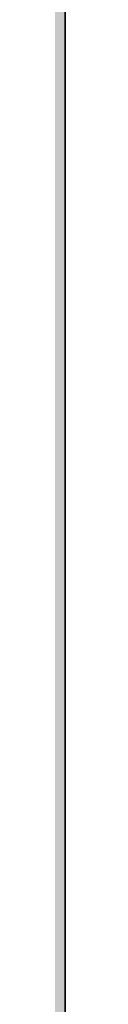
# Model space of a CAD drawing. Units: inches. Extents: x 2091 to 2899, y 967 to 2217.
# Tile 56 of 256: x 2212.14352 to 2212.1436, y 1099.95712 to 1099.99878. Entities that reach past the tile are written whole.
import ezdxf

# ---------------------------------------------------------------- set-up
doc = ezdxf.new("R2010")
doc.units = ezdxf.units.IN
doc.layers.add('A-WALL', color=7, linetype='Continuous', lineweight=35)
doc.layers.add('A-WALL-PATT', color=141, linetype='Continuous', lineweight=13, true_color=0xadddf7)

msp = doc.modelspace()

# ---------------------------------------------------------------- hatches: boundary and pattern name
at = {"layer": 'A-WALL-PATT'}
h = msp.add_hatch(color=256, dxfattribs=at)
h.dxf.hatch_style = 1
h.paths.add_polyline_path([(2212.143603, 1941.419059), (2387.643603, 1941.419059), (2387.643603, 1824.419059), (2392.143603, 1824.419059), (2392.143603, 1941.419059), (2609.643603, 1941.419059), (2609.643603, 1825.919059), (2614.143603, 1825.919059), (2614.143603, 1941.419059), (2794.143603, 1941.419059), (2794.143603, 1928.762166), (2803.143603, 1928.762166), (2803.143603, 2050.919059), (2203.143603, 2050.919059), (2203.143603, 1900.757859), (2212.143603, 1900.757859)])
h.paths.add_polyline_path([(2212.143603, 1945.919059), (2212.143603, 2041.919059), (2794.143603, 2041.919059), (2794.143603, 1945.919059), (2402.248245, 1945.919059), (2401.102434, 1945.775832), (2398.702434, 1945.775832)], flags=16)
h.paths.add_polyline_path([(2230.229861, 1948.062793), (2227.349861, 1949.502793), (2225.909861, 1951.902793), (2223.989861, 1952.862793), (2223.029861, 1955.262793), (2222.069861, 1959.582793), (2222.069861, 1963.422793), (2223.029861, 1965.662793), (2223.989861, 1965.342793), (2225.58591, 1963.860747), (2226.911533, 1964.957259), (2226.948861, 1965.938793), (2227.778319, 1966.952143), (2228.199916, 1968.878704), (2230.709861, 1964.862793), (2233.589861, 1966.302793), (2233.607309, 1966.331873), (2233.772659, 1964.938205), (2234.633802, 1963.676473), (2235.029861, 1963.902793), (2236.282035, 1965.572358), (2235.989861, 1962.942793), (2237.954512, 1957.540002), (2238.389861, 1957.902793), (2239.215861, 1960.305793), (2238.654565, 1966.38496), (2238.692792, 1966.438069), (2238.840578, 1967.499707), (2238.780291, 1967.687486), (2238.880538, 1967.786763), (2238.666861, 1966.251793), (2239.215861, 1960.305793), (2238.389861, 1957.902793), (2236.949861, 1956.702793), (2234.549861, 1949.982793)], flags=0)
h.paths.add_polyline_path([(2278.011974, 1948.062793), (2276.496427, 1947.873349), (2275.849833, 1947.688608), (2274.651974, 1947.102793)], flags=0)
h.paths.add_polyline_path([(2269.851974, 1955.742793), (2268.276176, 1956.629329), (2270.867302, 1956.348398), (2269.371974, 1958.142793), (2268.714964, 1959.192325), (2270.569833, 1958.728608), (2268.580725, 1961.906087), (2270.811974, 1960.891883), (2270.811974, 1963.422793), (2271.393315, 1964.779256), (2270.291762, 1966.156196), (2271.771974, 1965.662793), (2272.141387, 1966.524757), (2273.929833, 1965.928608), (2275.630385, 1968.054299), (2276.331938, 1966.72186), (2276.520431, 1966.952143), (2276.942029, 1968.878704), (2277.734293, 1967.611082), (2278.139888, 1969.46452), (2279.659124, 1967.033742), (2280.411974, 1966.782793), (2280.949302, 1967.588785), (2281.609833, 1967.368608), (2282.133266, 1968.153758), (2282.349235, 1966.333445), (2282.349849, 1966.332585), (2283.40755, 1968.09542), (2283.712631, 1965.52402), (2284.320221, 1964.633789), (2284.511809, 1964.889239), (2284.234974, 1965.704793), (2284.500472, 1967.318958), (2284.907944, 1965.41742), (2285.396313, 1966.068579), (2285.432833, 1966.290608), (2285.473338, 1966.171279), (2286.353919, 1967.345387), (2286.222007, 1966.158173), (2287.663492, 1968.080154), (2287.713974, 1968.442793), (2288.481599, 1969.016679), (2288.573993, 1968.728897), (2288.917461, 1969.06904), (2288.606833, 1966.837608), (2288.928726, 1963.35131), (2288.934974, 1963.356793), (2288.929731, 1963.340422), (2289.015281, 1962.413869), (2290.111223, 1963.875126), (2290.132833, 1963.942608), (2290.217672, 1964.017058), (2290.111223, 1963.875126), (2289.155833, 1960.891608), (2288.594036, 1959.257227), (2288.571974, 1959.102793), (2289.531974, 1960.542793), (2290.011974, 1962.462793), (2290.19184, 1962.642659), (2289.769833, 1959.688608), (2286.889833, 1957.288608), (2284.489833, 1950.568608), (2283.314658, 1950.046308), (2283.291974, 1949.982793), (2280.290059, 1948.648608), (2281.129833, 1948.648608), (2282.569833, 1948.168608), (2283.204726, 1948.062793), (2278.971974, 1948.062793), (2276.091974, 1949.502793), (2274.651974, 1951.902793), (2272.731974, 1952.862793)], flags=0)
h.paths.add_polyline_path([(2271.158868, 1958.021765), (2272.969833, 1955.848608), (2272.009833, 1960.168608), (2272.009833, 1964.008608), (2272.624426, 1965.442658), (2274.328023, 1963.860747), (2275.653646, 1964.957259), (2275.637743, 1964.53909), (2277.412231, 1966.006888), (2277.032974, 1965.156793), (2276.829924, 1964.975597), (2276.766012, 1963.295014), (2277.449635, 1962.66022), (2279.451974, 1964.862793), (2282.331974, 1966.302793), (2283.529833, 1966.888608), (2283.294512, 1966.770948), (2283.912993, 1963.8847), (2284.899249, 1964.448275), (2284.731974, 1962.942793), (2286.696625, 1957.540002), (2287.131974, 1957.902793), (2287.541913, 1959.095388), (2287.779395, 1958.442311), (2285.682738, 1956.695097), (2285.876503, 1959.795336), (2284.731974, 1962.942793), (2284.899249, 1964.448275), (2283.912993, 1963.8847), (2284.223833, 1962.434116), (2283.424365, 1963.605484), (2281.609833, 1962.568608), (2281.129833, 1960.168608), (2282.089833, 1956.328608), (2283.049833, 1952.968608), (2282.569833, 1950.568608), (2280.169833, 1948.648608), (2279.883316, 1948.791867), (2278.971974, 1948.062793), (2278.971974, 1949.022793), (2278.672313, 1949.397368), (2277.289833, 1950.088608), (2275.849833, 1952.488608), (2273.929833, 1953.448608), (2272.489833, 1954.888608), (2271.921647, 1954.888608), (2271.771974, 1955.262793)], flags=0)
h.paths.add_polyline_path([(2311.994146, 1955.742793), (2312.062717, 1955.674221), (2312.0551, 1955.7085)], flags=0)
h.paths.add_polyline_path([(2331.956146, 1963.951793), (2333.396146, 1965.391793), (2331.077146, 1963.356793), (2330.998603, 1963.111517)], flags=0)
h.paths.add_polyline_path([(2310.554146, 1954.302793), (2307.039807, 1956.279943), (2310.762903, 1955.876284), (2312.474146, 1953.822793), (2313.434146, 1951.422793), (2315.354146, 1950.462793), (2316.794146, 1948.062793), (2317.466146, 1947.726793), (2319.368691, 1947.964611), (2317.754146, 1949.982793), (2317.569531, 1950.610485), (2316.794146, 1951.902793), (2314.874146, 1952.862793), (2313.914146, 1955.262793), (2311.514146, 1958.142793), (2309.375489, 1961.559168), (2311.514146, 1960.337078), (2311.514146, 1961.982793), (2310.604672, 1963.119635), (2311.726605, 1962.47853), (2312.418332, 1964.09256), (2312.255964, 1964.29552), (2313.194146, 1963.982793), (2313.914146, 1965.662793), (2314.646778, 1965.418582), (2315.354146, 1966.302793), (2316.794146, 1967.742793), (2316.157435, 1966.946904), (2317.034111, 1965.28186), (2317.222604, 1965.512143), (2317.777048, 1968.045771), (2318.474111, 1966.72186), (2318.662604, 1966.952143), (2319.084201, 1968.878704), (2321.207049, 1965.482147), (2322.161419, 1966.913702), (2322.554146, 1966.782793), (2322.785988, 1967.130555), (2322.881646, 1966.324293), (2323.312041, 1965.72174), (2323.651289, 1965.891364), (2324.3965, 1967.133382), (2324.656945, 1964.938205), (2324.971986, 1964.476611), (2325.38728, 1967.001499), (2325.940813, 1964.418348), (2327.228929, 1966.135836), (2327.16632, 1965.572358), (2328.059139, 1966.762783), (2328.224576, 1966.247486), (2329.667971, 1967.67691), (2329.664576, 1967.687486), (2329.764823, 1967.786763), (2329.551146, 1966.251793), (2330.100146, 1960.305793), (2329.332814, 1958.07347), (2329.313065, 1957.935225), (2329.634146, 1958.202793), (2330.234146, 1959.102793), (2330.714146, 1961.022793), (2331.034146, 1961.342793), (2330.714146, 1959.102793), (2329.634146, 1958.202793), (2329.274146, 1957.662793), (2327.712112, 1956.361098), (2325.434146, 1949.982793), (2324.333769, 1949.493736), (2323.994146, 1948.542793), (2319.674146, 1946.622793), (2316.794146, 1948.062793), (2315.354146, 1950.462793), (2313.434146, 1951.422793)], flags=0)
h.paths.add_polyline_path([(2321.335684, 1947.952023), (2321.114146, 1948.062793), (2321.114146, 1949.022793), (2319.194146, 1951.422793), (2316.794146, 1959.582793), (2316.663237, 1959.582793), (2315.354146, 1958.142793), (2314.394146, 1958.142793), (2313.148303, 1958.709085), (2312.954146, 1959.582793), (2312.954146, 1960.891883), (2315.834146, 1959.582793), (2316.663237, 1959.582793), (2317.314709, 1960.299412), (2315.030195, 1962.420747), (2316.355818, 1963.517259), (2316.372337, 1963.951615), (2316.470195, 1963.860747), (2317.795818, 1964.957259), (2317.755219, 1963.889687), (2319.175146, 1965.156793), (2319.498407, 1965.881372), (2321.114146, 1965.342793), (2323.235885, 1962.372358), (2325.686349, 1963.772623), (2325.542789, 1962.480576), (2325.198783, 1963.494014), (2324.47851, 1963.082429), (2324.926005, 1960.994116), (2324.078087, 1962.236473), (2322.414791, 1961.286018), (2322.074146, 1959.582793), (2323.034146, 1955.742793), (2323.994146, 1952.382793), (2323.514146, 1949.982793), (2322.142717, 1948.88565), (2322.074146, 1948.542793)], flags=0)
h.paths.add_polyline_path([(2320.207479, 1963.337459), (2320.154146, 1963.422793), (2320.394146, 1963.542793)], flags=0)
h.paths.add_polyline_path([(2353.850527, 1965.8105), (2354.030527, 1965.7505), (2354.330527, 1966.4505), (2354.330527, 1966.9305)], flags=0)
h.paths.add_polyline_path([(2359.020582, 1969.026412), (2359.098382, 1968.901932), (2359.233527, 1969.5195), (2359.233527, 1969.9995)], flags=0)
h.paths.add_polyline_path([(2358.256694, 1966.681672), (2357.983601, 1966.348035), (2358.211267, 1966.146175), (2358.410492, 1966.389568)], flags=0)
h.paths.add_polyline_path([(2357.768473, 1966.058778), (2357.7322, 1965.104967), (2357.751047, 1965.120556), (2357.769527, 1965.6065), (2357.769527, 1966.057843)], flags=0)
h.paths.add_polyline_path([(2359.111527, 1965.3045), (2359.111527, 1964.8245), (2359.844527, 1966.4675), (2359.844527, 1966.9475)], flags=0)
h.paths.add_polyline_path([(2360.223684, 1966.621449), (2360.698527, 1969.3625), (2360.698527, 1969.8425), (2360.210527, 1967.0255), (2360.210527, 1966.6425)], flags=0)
h.paths.add_polyline_path([(2363.450527, 1967.8905), (2363.450527, 1968.3705), (2362.490527, 1966.9305), (2362.656045, 1966.698776)], flags=0)
h.paths.add_polyline_path([(2364.475523, 1966.078826), (2365.850527, 1968.3705), (2365.850527, 1968.8505), (2364.427975, 1966.479581)], flags=0)
h.paths.add_polyline_path([(2366.313527, 1965.8525), (2366.366709, 1965.695829), (2366.802527, 1968.3455), (2366.802527, 1968.8255)], flags=0)
h.paths.add_polyline_path([(2367.16531, 1965.803544), (2367.290527, 1966.9305), (2367.290527, 1967.4105), (2367.102701, 1965.720066)], flags=0)
h.paths.add_polyline_path([(2370.036527, 1959.9735), (2371.013527, 1963.0245), (2371.013527, 1963.5045), (2370.036527, 1960.4535)], flags=0)
h.paths.add_polyline_path([(2371.610527, 1960.2105), (2372.570527, 1961.6505), (2372.570527, 1962.1305), (2371.802527, 1960.9785)], flags=0)
h.paths.add_polyline_path([(2350.873666, 1956.005086), (2351.930527, 1955.8905), (2354.490527, 1953.3305), (2353.850527, 1954.9305), (2351.450527, 1957.8105), (2347.935527, 1963.4255), (2347.935527, 1963.9055), (2351.450527, 1958.2905), (2353.705073, 1955.585046), (2352.890527, 1959.2505), (2352.890527, 1959.7305), (2352.890527, 1961.924786), (2356.730527, 1959.7305), (2358.454471, 1961.626838), (2354.810527, 1965.0105), (2355.030855, 1965.28591), (2358.691091, 1961.88712), (2361.530527, 1965.0105), (2364.376495, 1966.433484), (2364.524394, 1965.186911), (2365.454468, 1963.824181), (2365.881073, 1964.067955), (2365.370527, 1966.4505), (2365.370527, 1966.9305), (2366.810527, 1960.2105), (2366.810527, 1959.7305), (2366.388709, 1952.981409), (2367.770527, 1956.8505), (2368.641225, 1957.576082), (2366.810527, 1962.6105), (2366.810527, 1963.0905), (2368.775179, 1957.68771), (2369.210527, 1958.0505), (2370.001592, 1960.351867), (2369.475232, 1966.052668), (2369.513458, 1966.105777), (2369.514173, 1966.110912), (2369.475232, 1966.532668), (2369.513458, 1966.585777), (2369.614635, 1967.312591), (2369.182527, 1968.6585), (2369.182527, 1969.1385), (2369.600957, 1967.835194), (2369.701204, 1967.934471), (2369.717947, 1968.054743), (2370.145176, 1968.374145), (2369.778707, 1968.011224), (2369.701204, 1967.454471), (2370.468161, 1968.214004), (2369.674936, 1967.265771), (2369.514173, 1966.110912), (2370.036527, 1960.4535), (2370.036527, 1959.9735), (2369.441756, 1958.243191), (2370.650527, 1959.2505), (2371.045821, 1962.017559), (2371.130527, 1962.1305), (2370.650527, 1958.7705), (2367.770527, 1956.3705), (2365.370527, 1949.6505), (2362.079099, 1948.187643), (2363.450527, 1947.7305), (2361.050527, 1947.7305), (2360.090527, 1947.7305), (2357.103861, 1947.357167), (2360.090527, 1948.2105), (2358.170527, 1949.1705), (2356.730527, 1951.5705), (2354.810527, 1952.5305), (2351.930527, 1955.4105)], flags=0)
h.paths.add_polyline_path([(2361.050527, 1948.6905), (2359.130527, 1951.0905), (2356.730527, 1959.2505), (2355.770527, 1959.2505), (2352.890527, 1960.559591), (2352.890527, 1961.444786), (2355.890527, 1959.7305), (2356.730527, 1959.7305), (2356.837194, 1959.367834), (2361.530527, 1964.5305), (2363.248422, 1965.389448), (2364.92531, 1963.041805), (2362.490527, 1961.6505), (2362.063861, 1959.517167), (2362.970527, 1955.8905), (2363.930527, 1952.5305), (2363.930527, 1952.0505), (2363.450527, 1949.6505), (2361.050527, 1947.7305)], flags=0)
h.paths.add_polyline_path([(2359.130527, 1951.5705), (2359.290527, 1951.3705), (2361.050527, 1954.4505), (2361.050527, 1954.9305)], flags=0)
h.paths.add_polyline_path([(2357.219527, 1966.5455), (2356.792527, 1968.8145), (2356.792527, 1969.2945), (2357.219527, 1967.0255)], flags=0)
h.paths.add_polyline_path([(2361.050527, 1954.4505), (2361.530527, 1958.7705), (2361.530527, 1959.2505), (2361.050527, 1954.9305)], flags=0)
h.paths.add_polyline_path([(2402.548287, 1948.486076), (2402.302434, 1948.415832), (2402.590434, 1948.415832)], flags=0)
h.paths.add_polyline_path([(2394.142434, 1956.095832), (2395.685052, 1954.553214), (2396.720495, 1953.970679), (2396.062434, 1955.615832), (2395.241381, 1956.601096), (2395.878904, 1956.441715), (2395.102434, 1959.935832), (2395.102434, 1963.775832), (2396.062434, 1966.015832), (2397.022434, 1965.695832), (2398.618483, 1964.213787), (2399.944106, 1965.310299), (2399.981434, 1966.291832), (2400.810891, 1967.305183), (2401.232489, 1969.231744), (2403.537949, 1965.543008), (2403.941984, 1967.389316), (2404.702434, 1967.135832), (2405.460328, 1966.07478), (2406.622434, 1966.655832), (2406.639882, 1966.684913), (2406.805232, 1965.291245), (2406.925694, 1965.114746), (2407.342434, 1964.975832), (2407.874326, 1965.77367), (2408.1691, 1964.398055), (2409.314608, 1965.925398), (2409.217458, 1965.051054), (2409.445232, 1963.131245), (2410.306374, 1961.869513), (2410.702434, 1962.095832), (2411.442269, 1963.082279), (2411.165434, 1963.897832), (2411.616426, 1966.639757), (2411.725365, 1966.791109), (2411.873151, 1967.852747), (2411.812864, 1968.040526), (2411.913111, 1968.139803), (2411.699434, 1966.604832), (2412.248434, 1960.658832), (2413.225434, 1963.709832), (2414.3779, 1964.72116), (2414.513151, 1965.692747), (2414.452864, 1965.880526), (2414.553111, 1965.979803), (2414.3779, 1964.72116), (2414.519817, 1964.845697), (2414.365365, 1964.631109), (2414.339434, 1964.444832), (2414.888434, 1958.498832), (2414.062434, 1956.095832), (2412.622434, 1954.895832), (2410.17137, 1948.032854), (2410.016719, 1948.084404), (2405.902434, 1946.255832), (2405.902434, 1947.215832), (2405.204252, 1948.08856), (2404.222434, 1948.415832), (2403.262434, 1948.415832), (2400.382434, 1949.855832), (2399.662434, 1951.055832), (2397.982434, 1952.735832), (2397.022434, 1953.215832), (2395.685052, 1954.553214), (2392.656776, 1956.256908)], flags=0)
h.paths.add_polyline_path([(2409.08565, 1964.407441), (2409.130363, 1964.275715), (2409.262434, 1964.495832)], flags=0)
h.paths.add_polyline_path([(2397.742434, 1961.615832), (2398.702434, 1963.855832), (2399.662434, 1963.535832), (2401.426563, 1965.740994), (2401.791415, 1966.5588), (2402.071434, 1965.070832), (2402.835507, 1964.393367), (2403.262398, 1964.9149), (2403.338119, 1964.771086), (2402.615516, 1963.976223), (2402.498612, 1960.902238), (2403.542997, 1959.932452), (2404.413203, 1960.889679), (2404.702434, 1962.335832), (2407.916347, 1964.172354), (2409.520211, 1961.926944), (2410.987085, 1957.893042), (2411.422434, 1958.255832), (2412.047964, 1960.075625), (2412.410341, 1959.079088), (2411.675621, 1958.466821), (2411.662434, 1958.255832), (2411.62607, 1958.425529), (2409.982434, 1957.055832), (2407.582434, 1950.335832), (2403.262434, 1948.415832), (2403.262434, 1949.375832), (2401.342434, 1951.775832), (2399.416508, 1958.323981), (2397.742434, 1959.084923), (2397.742434, 1959.970118), (2397.102434, 1960.335832), (2397.742434, 1960.044923)], flags=0)
h.paths.add_polyline_path([(2405.902434, 1952.975832), (2405.950434, 1953.407832), (2406.016719, 1953.175832)], flags=0)
h.paths.add_polyline_path([(2449.817778, 1967.114014), (2449.752323, 1967.135832), (2449.793703, 1967.077901)], flags=0)
h.paths.add_polyline_path([(2451.697696, 1966.61812), (2451.740895, 1966.690118), (2451.692051, 1966.665696)], flags=0)
h.paths.add_polyline_path([(2454.343628, 1965.737572), (2455.752323, 1967.615832), (2455.992323, 1968.095832), (2454.364497, 1965.925398)], flags=0)
h.paths.add_polyline_path([(2457.547323, 1968.863832), (2457.787323, 1969.343832), (2457.054323, 1968.795832), (2457.007622, 1968.460345)], flags=0)
h.paths.add_polyline_path([(2456.921784, 1967.856662), (2456.802238, 1968.229016), (2456.723, 1967.659803)], flags=0)
h.paths.add_polyline_path([(2457.302323, 1967.376832), (2457.542323, 1967.856832), (2456.810323, 1966.839832), (2456.740516, 1966.700218), (2456.749021, 1966.608105)], flags=0)
h.paths.add_polyline_path([(2458.275323, 1963.709832), (2458.155343, 1963.335153), (2460.354323, 1965.264832), (2460.594323, 1965.744832)], flags=0)
h.paths.add_polyline_path([(2458.392323, 1962.815832), (2458.364088, 1962.618185), (2459.592323, 1964.255832), (2459.832323, 1964.735832)], flags=0)
h.paths.add_polyline_path([(2459.352323, 1962.815832), (2459.272323, 1962.495832), (2460.072323, 1963.295832), (2460.312323, 1963.775832)], flags=0)
h.paths.add_polyline_path([(2458.680323, 1960.607832), (2458.632323, 1960.415832), (2459.592323, 1961.855832), (2459.832323, 1962.335832)], flags=0)
h.paths.add_polyline_path([(2437.83817, 1956.24265), (2439.192323, 1956.095832), (2441.352323, 1953.935832), (2440.872323, 1955.135832), (2438.472323, 1958.015832), (2438.071563, 1958.656023), (2438.712323, 1958.495832), (2440.639596, 1956.183105), (2439.912323, 1959.455832), (2439.912323, 1963.295832), (2441.352323, 1966.655832), (2441.592323, 1967.135832), (2441.112323, 1966.015832), (2442.072323, 1965.695832), (2443.988993, 1968.09167), (2444.241323, 1966.750832), (2444.916801, 1966.15192), (2445.676574, 1967.080136), (2446.255323, 1969.724832), (2446.495323, 1970.204832), (2446.282379, 1969.231744), (2447.362672, 1967.503275), (2447.720323, 1969.567832), (2447.960323, 1970.047832), (2447.48548, 1967.306781), (2448.792323, 1965.215832), (2448.472323, 1964.863832), (2448.552323, 1964.735832), (2451.452051, 1966.185696), (2451.615122, 1964.811245), (2452.307917, 1963.796172), (2453.234505, 1964.325651), (2454.072323, 1960.415832), (2453.628687, 1953.317651), (2454.792323, 1956.575832), (2455.032323, 1957.055832), (2455.718835, 1957.627926), (2453.832323, 1962.815832), (2453.940966, 1963.793615), (2453.335323, 1965.577832), (2453.824323, 1968.550832), (2454.064323, 1969.030832), (2453.575323, 1966.057832), (2454.040333, 1964.687919), (2453.832323, 1962.815832), (2455.718835, 1957.627926), (2456.367207, 1958.168235), (2457.058323, 1960.178832), (2457.298323, 1960.658832), (2456.472323, 1958.255832), (2457.717729, 1959.29367), (2457.672323, 1958.975832), (2454.889951, 1956.657188), (2453.614142, 1953.084923), (2453.592323, 1952.735832), (2453.352323, 1952.255832), (2453.359596, 1952.372196), (2452.632323, 1950.335832), (2452.392323, 1949.855832), (2449.203752, 1948.43869), (2450.712323, 1947.935832), (2448.072323, 1947.935832), (2447.112323, 1947.935832), (2444.552323, 1947.615832), (2447.199596, 1948.372196), (2445.192323, 1949.375832), (2443.752323, 1951.775832), (2441.832323, 1952.735832), (2438.952323, 1955.615832)], flags=0)
h.paths.add_polyline_path([(2443.992323, 1959.935832), (2444.040323, 1959.772632), (2444.121554, 1959.861986)], flags=0)
h.paths.add_polyline_path([(2442.912323, 1959.935832), (2443.032323, 1959.935832), (2442.445657, 1960.202499)], flags=0)
h.paths.add_polyline_path([(2444.982943, 1965.019677), (2445.279323, 1965.264832), (2445.519323, 1965.744832), (2444.993996, 1965.310299)], flags=0)
h.paths.add_polyline_path([(2446.133323, 1965.029832), (2446.330366, 1965.471499), (2444.970323, 1964.257832), (2444.730323, 1963.777832)], flags=0)
h.paths.add_polyline_path([(2442.792323, 1959.455832), (2443.752323, 1959.455832), (2446.152323, 1951.295832), (2446.412323, 1951.750832), (2446.392323, 1951.775832), (2448.080599, 1954.730315), (2448.552323, 1958.975832), (2441.832323, 1965.215832), (2442.154946, 1965.619111), (2448.792323, 1959.455832), (2448.312323, 1955.135832), (2448.072323, 1954.655832), (2446.412323, 1951.750832), (2448.312323, 1949.375832), (2448.312323, 1948.415832), (2450.540895, 1950.19869), (2450.952323, 1952.255832), (2449.992323, 1955.615832), (2449.032323, 1959.455832), (2449.512323, 1961.855832), (2449.752323, 1962.335832), (2449.674904, 1961.948736), (2452.994505, 1963.845651), (2453.064414, 1963.519409), (2452.884611, 1963.782854), (2449.674904, 1961.948736), (2449.272323, 1959.935832), (2450.232323, 1956.095832), (2451.192323, 1952.735832), (2450.712323, 1950.335832), (2450.472323, 1949.855832), (2448.072323, 1947.935832), (2448.072323, 1948.535832), (2445.432323, 1949.855832), (2443.992323, 1952.255832), (2442.072323, 1953.215832), (2441.112323, 1955.615832), (2440.152323, 1959.935832), (2440.152323, 1960.655832)], flags=0)
h.paths.add_polyline_path([(2456.692323, 1966.985832), (2457.608323, 1968.080832), (2457.848323, 1968.560832), (2456.932323, 1967.465832)], flags=0)
h.paths.add_polyline_path([(2489.89657, 1966.580241), (2489.942948, 1966.189347), (2490.747488, 1967.530248), (2491.319122, 1968.951161)], flags=0)
h.paths.add_polyline_path([(2473.562471, 1956.407131), (2477.139981, 1956.019257), (2476.955333, 1956.240834), (2475.108049, 1957.280108), (2476.347488, 1956.970248), (2475.186901, 1958.824216), (2476.919122, 1958.391161), (2475.411642, 1960.799269), (2477.787488, 1959.719339), (2477.787488, 1962.250248), (2477.637399, 1962.43786), (2477.82255, 1962.332059), (2478.359122, 1963.58406), (2478.359122, 1963.671161), (2477.324348, 1964.964628), (2478.714826, 1964.501135), (2479.319122, 1965.911161), (2480.279122, 1965.591161), (2481.783965, 1967.472214), (2482.116488, 1965.705248), (2482.880562, 1965.027782), (2483.209305, 1965.429408), (2483.220169, 1965.71509), (2483.07594, 1965.989022), (2483.711762, 1966.765808), (2484.130488, 1968.679248), (2484.702122, 1970.100161), (2484.489177, 1969.127072), (2486.502904, 1965.905109), (2487.387488, 1965.610248), (2488.153419, 1966.759144), (2488.717017, 1965.970108), (2489.200086, 1966.211642), (2489.330671, 1965.110992), (2490.393905, 1963.622465), (2490.660765, 1963.774956), (2490.493905, 1964.553636), (2490.923063, 1963.924841), (2491.319122, 1964.151161), (2491.333389, 1964.170183), (2491.210488, 1964.532248), (2491.281756, 1964.965537), (2491.425789, 1964.293383), (2494.076476, 1967.827632), (2494.497918, 1966.514942), (2494.598165, 1966.614218), (2494.689488, 1967.270248), (2495.106748, 1967.582196), (2495.129839, 1967.748075), (2495.069552, 1967.935854), (2495.169799, 1968.035131), (2495.031777, 1967.043632), (2495.753818, 1967.758684), (2494.982053, 1966.686437), (2494.956122, 1966.500161), (2495.479021, 1960.836851), (2495.910488, 1962.184248), (2496.482122, 1963.605161), (2496.072694, 1962.326589), (2496.768904, 1962.937536), (2496.599122, 1962.711161), (2496.119122, 1959.351161), (2496.732873, 1960.271787), (2496.987488, 1961.290248), (2497.559122, 1962.711161), (2497.079122, 1960.791161), (2496.507488, 1959.370248), (2495.547488, 1957.930248), (2492.758842, 1955.606376), (2490.839122, 1950.231161), (2490.267488, 1948.810248), (2485.947488, 1946.890248), (2483.067488, 1948.330248), (2481.627488, 1950.730248), (2479.707488, 1951.690248), (2476.827488, 1954.570248)], flags=0)
h.paths.add_polyline_path([(2485.576973, 1948.313392), (2485.559122, 1948.311161), (2485.578758, 1948.311161)], flags=0)
h.paths.add_polyline_path([(2478.645063, 1954.551161), (2478.109042, 1956.963257), (2479.319122, 1955.511161), (2480.279122, 1953.111161), (2482.199122, 1952.151161), (2483.639122, 1949.751161), (2486.519122, 1948.311161), (2486.519122, 1949.271161), (2484.739307, 1951.49593), (2484.027488, 1950.250248), (2481.627488, 1958.410248), (2482.375148, 1959.232673), (2482.199122, 1959.831161), (2483.197572, 1960.929456), (2479.707488, 1964.170248), (2480.603358, 1965.290085), (2481.875171, 1964.109115), (2482.666387, 1964.763582), (2482.615359, 1963.421798), (2482.989199, 1963.074661), (2484.008488, 1963.984248), (2484.683606, 1965.497507), (2484.580122, 1965.405161), (2485.357268, 1967.147113), (2485.120645, 1965.781197), (2486.427488, 1963.690248), (2488.145383, 1964.549195), (2489.822271, 1962.201552), (2490.747488, 1962.730248), (2491.999662, 1964.399813), (2492.076046, 1965.087265), (2492.212892, 1964.684119), (2492.485374, 1965.047429), (2492.279122, 1963.191161), (2494.243773, 1957.78837), (2494.562503, 1958.053978), (2494.933488, 1959.133248), (2495.505122, 1960.554161), (2494.679122, 1958.151161), (2494.107488, 1956.730248), (2494.562503, 1958.053978), (2493.408544, 1957.092345), (2491.707488, 1961.770248), (2491.999662, 1964.399813), (2490.747488, 1962.730248), (2487.71203, 1960.9957), (2487.479122, 1959.831161), (2488.439122, 1955.991161), (2489.399122, 1952.631161), (2488.919122, 1950.231161), (2488.576918, 1949.957397), (2488.347488, 1948.810248), (2487.651715, 1948.253629), (2487.479122, 1948.311161), (2486.519122, 1948.311161), (2483.639122, 1949.751161), (2482.199122, 1952.151161), (2480.279122, 1953.111161), (2478.839122, 1954.551161)], flags=0)
h.paths.add_polyline_path([(2526.648252, 1966.987524), (2526.517343, 1967.031161), (2526.600102, 1966.915298)], flags=0)
h.paths.add_polyline_path([(2528.47064, 1966.446656), (2528.574486, 1966.619732), (2528.457071, 1966.561025)], flags=0)
h.paths.add_polyline_path([(2534.133343, 1967.496161), (2534.156685, 1967.542845), (2534.059841, 1967.408296)], flags=0)
h.paths.add_polyline_path([(2536.161923, 1964.0506), (2535.157343, 1962.711161), (2535.100872, 1962.315866), (2536.117343, 1963.671161), (2536.420532, 1964.277539)], flags=0)
h.paths.add_polyline_path([(2535.157343, 1959.831161), (2536.117343, 1961.271161), (2536.597343, 1962.231161), (2535.253343, 1960.215161)], flags=0)
h.paths.add_polyline_path([(2513.249035, 1956.284796), (2516.221181, 1955.962555), (2514.997343, 1957.431161), (2514.195823, 1958.711541), (2515.477343, 1958.391161), (2516.931888, 1956.645706), (2516.437343, 1958.871161), (2516.437343, 1962.711161), (2516.872692, 1963.726974), (2515.346434, 1965.634797), (2517.397343, 1964.951161), (2517.877343, 1966.071161), (2518.357343, 1967.031161), (2517.877343, 1965.911161), (2518.837343, 1965.591161), (2520.48659, 1967.652719), (2520.766343, 1966.166161), (2521.530417, 1965.488695), (2521.781443, 1965.795375), (2521.800911, 1966.307268), (2521.477804, 1966.920936), (2521.246343, 1967.126161), (2521.177701, 1967.490913), (2521.477804, 1966.920936), (2522.010417, 1966.448695), (2522.257386, 1966.750417), (2522.780343, 1969.140161), (2523.260343, 1970.100161), (2523.047398, 1969.127072), (2524.673132, 1966.525897), (2526.037343, 1966.071161), (2526.795238, 1965.010108), (2527.977071, 1965.601025), (2528.140141, 1964.226573), (2528.66459, 1963.458159), (2529.388616, 1963.871888), (2529.329665, 1964.14699), (2529.481284, 1963.924841), (2529.877343, 1964.151161), (2529.98401, 1964.293383), (2529.789053, 1965.20318), (2530.0624, 1964.397903), (2532.802483, 1968.051347), (2533.147773, 1966.975854), (2533.24802, 1967.075131), (2533.339343, 1967.731161), (2533.672848, 1967.980493), (2533.72802, 1968.035131), (2533.514343, 1966.500161), (2534.024718, 1960.972496), (2534.560343, 1962.645161), (2535.040343, 1963.605161), (2534.063343, 1960.554161), (2533.237343, 1958.151161), (2534.288154, 1959.026836), (2534.197343, 1958.391161), (2531.512597, 1956.153872), (2529.397343, 1950.231161), (2528.917343, 1949.271161), (2526.448772, 1948.174018), (2527.477343, 1947.831161), (2530.357343, 1947.351161), (2524.597343, 1947.351161), (2521.717343, 1948.791161), (2520.277343, 1951.191161), (2518.357343, 1952.151161), (2515.477343, 1955.031161)], flags=0)
h.paths.add_polyline_path([(2523.93476, 1967.190308), (2523.619512, 1966.483689), (2523.7705, 1966.242109)], flags=0)
h.paths.add_polyline_path([(2518.837343, 1953.111161), (2517.877343, 1955.511161), (2516.884983, 1959.976779), (2516.917343, 1959.96207), (2516.917343, 1962.025446), (2520.757343, 1959.831161), (2522.024949, 1961.225527), (2518.357343, 1964.631161), (2519.002589, 1965.437718), (2520.433392, 1964.109115), (2521.30112, 1964.826871), (2521.245157, 1963.355333), (2525.638307, 1959.27598), (2526.037343, 1961.271161), (2529.397343, 1963.191161), (2530.649517, 1964.860726), (2530.66472, 1964.99755), (2530.691956, 1964.917311), (2531.087778, 1965.445074), (2530.945985, 1964.168944), (2530.691956, 1964.917311), (2529.397343, 1963.191161), (2526.362504, 1961.456967), (2526.037343, 1959.831161), (2526.997343, 1955.991161), (2527.957343, 1952.631161), (2527.477343, 1950.231161), (2527.134486, 1949.956875), (2526.973928, 1949.154087), (2526.697343, 1949.031161), (2524.597343, 1947.351161), (2524.597343, 1948.311161), (2524.277343, 1948.711161), (2522.197343, 1949.751161), (2520.757343, 1952.151161)], flags=0)
h.paths.add_polyline_path([(2520.277343, 1958.871161), (2520.853343, 1959.504761), (2523.157343, 1951.671161), (2524.613895, 1954.220126), (2524.597343, 1954.071161), (2522.677343, 1950.711161)], flags=0)
h.paths.add_polyline_path([(2559.37091, 1966.311161), (2559.398411, 1966.324911), (2559.401943, 1966.345296)], flags=0)
h.paths.add_polyline_path([(2549.77091, 1957.191161), (2552.65091, 1954.311161), (2552.133987, 1955.603468), (2550.61091, 1957.431161), (2547.09591, 1963.046161), (2545.77591, 1965.206161), (2549.29091, 1959.591161), (2551.69091, 1956.711161), (2550.792933, 1960.752059), (2550.73091, 1960.780251), (2550.73091, 1964.871161), (2551.69091, 1967.111161), (2552.65091, 1966.791161), (2554.246959, 1965.309115), (2555.034252, 1965.960337), (2555.581671, 1966.644612), (2555.60991, 1967.387161), (2556.439368, 1968.400511), (2556.860966, 1970.327072), (2559.37091, 1966.311161), (2560.69091, 1964.151161), (2562.408805, 1965.010108), (2561.65091, 1966.071161), (2560.33091, 1968.231161), (2561.758497, 1966.23254), (2562.347213, 1967.115614), (2562.433709, 1966.386573), (2563.127798, 1965.369604), (2563.57091, 1965.591161), (2563.588359, 1965.620241), (2563.362543, 1967.52354), (2563.722489, 1965.843792), (2565.060001, 1968.072979), (2564.732862, 1965.128722), (2565.117577, 1963.333383), (2567.444622, 1966.436109), (2567.315615, 1967.833328), (2567.353841, 1967.886437), (2567.501627, 1968.948075), (2567.44134, 1969.135854), (2567.541587, 1969.235131), (2567.32791, 1967.700161), (2567.87691, 1961.754161), (2568.746689, 1964.470327), (2568.635615, 1965.673328), (2568.673841, 1965.726437), (2568.821627, 1966.788075), (2568.76134, 1966.975854), (2568.861587, 1967.075131), (2568.64791, 1965.540161), (2568.726127, 1964.693026), (2568.85391, 1964.805161), (2568.746689, 1964.470327), (2568.817236, 1963.706261), (2568.97091, 1963.911161), (2568.866075, 1963.17731), (2569.19691, 1959.594161), (2568.37091, 1957.191161), (2566.93091, 1955.991161), (2564.620272, 1949.521373), (2564.65091, 1949.511161), (2564.616625, 1949.511161), (2564.53091, 1949.271161), (2560.21091, 1947.351161), (2557.33091, 1948.791161), (2556.045196, 1950.934018), (2556.01091, 1950.951161), (2555.856625, 1951.208303), (2553.97091, 1952.151161), (2551.09091, 1955.031161), (2546.650144, 1957.529515)], flags=0)
h.paths.add_polyline_path([(2567.025794, 1959.33023), (2567.035007, 1959.304895), (2567.05091, 1959.351161)], flags=0)
h.paths.add_polyline_path([(2551.968287, 1962.518374), (2553.01091, 1964.951161), (2553.97091, 1964.631161), (2555.566959, 1963.149115), (2556.892583, 1964.245627), (2556.92991, 1965.227161), (2557.143984, 1965.488695), (2556.420066, 1966.130557), (2556.391421, 1966.104995), (2556.37991, 1966.166161), (2556.420066, 1966.130557), (2556.95191, 1966.605161), (2557.092139, 1966.919478), (2557.570875, 1966.010228), (2557.759368, 1966.240511), (2557.41791, 1964.680161), (2556.892583, 1964.245627), (2556.807089, 1961.997566), (2560.69091, 1958.391161), (2560.635526, 1957.892699), (2560.81091, 1957.191161), (2561.77091, 1953.831161), (2561.29091, 1951.431161), (2559.110423, 1949.68677), (2559.156484, 1949.629193), (2563.02652, 1951.349209), (2562.61091, 1949.271161), (2560.21091, 1947.351161), (2560.21091, 1948.311161), (2559.25091, 1949.511161), (2558.89091, 1949.511161), (2558.89091, 1949.961161), (2558.29091, 1950.711161), (2558.053701, 1951.517672), (2556.97091, 1952.871161), (2555.06788, 1959.341464), (2552.05091, 1961.065446), (2552.05091, 1962.471161)], flags=0)
h.paths.add_polyline_path([(2588.330049, 1958.391161), (2588.610248, 1958.110962), (2588.553362, 1958.366949)], flags=0)
h.paths.add_polyline_path([(2594.745454, 1950.493086), (2593.957532, 1953.172022), (2593.130049, 1954.551161), (2591.210049, 1955.511161), (2590.250049, 1957.911161), (2588.309033, 1960.240379), (2586.177306, 1961.209346), (2587.850049, 1960.791161), (2587.253416, 1961.744246), (2588.441314, 1961.065446), (2588.441314, 1962.655528), (2588.421679, 1962.665345), (2588.441314, 1962.711161), (2586.914038, 1964.620256), (2588.877086, 1963.727962), (2589.290049, 1964.69154), (2589.290049, 1966.071161), (2590.250049, 1968.311161), (2591.210049, 1967.991161), (2592.806098, 1966.509115), (2594.131721, 1967.605627), (2594.169049, 1968.587161), (2594.998506, 1969.600511), (2595.420104, 1971.527072), (2597.930049, 1967.511161), (2600.810049, 1968.951161), (2600.827497, 1968.980241), (2600.992847, 1967.586573), (2601.853989, 1966.324841), (2602.107143, 1966.4695), (2602.236354, 1967.255069), (2602.356715, 1966.693383), (2603.502223, 1968.220726), (2603.210049, 1965.591161), (2605.1747, 1960.18837), (2605.506891, 1960.465196), (2605.026019, 1965.673328), (2605.064245, 1965.726437), (2605.212031, 1966.788075), (2605.151744, 1966.975854), (2605.251991, 1967.075131), (2605.343314, 1967.731161), (2605.952905, 1968.186898), (2605.874753, 1969.033328), (2605.912979, 1969.086437), (2606.060766, 1970.148075), (2606.000479, 1970.335854), (2606.100725, 1970.435131), (2605.887049, 1968.900161), (2606.436049, 1962.954161), (2605.610049, 1960.551161), (2605.997036, 1960.87365), (2606.564314, 1962.645161), (2608.241494, 1964.116941), (2608.010049, 1963.191161), (2607.050049, 1961.751161), (2606.631486, 1961.402358), (2606.201314, 1958.391161), (2603.321314, 1955.991161), (2600.921314, 1949.271161), (2596.601314, 1947.351161), (2593.721314, 1948.791161), (2592.857314, 1950.231161), (2592.650049, 1950.231161)], flags=0)
h.paths.add_polyline_path([(2596.601314, 1947.351161), (2596.601314, 1948.311161), (2594.681314, 1950.711161), (2596.154954, 1953.290029), (2595.530049, 1954.071161), (2593.199226, 1961.995957), (2592.65134, 1962.504708), (2591.780151, 1963.002531), (2593.282987, 1964.245627), (2593.320314, 1965.227161), (2594.149772, 1966.240511), (2594.57137, 1968.167072), (2596.182651, 1965.589023), (2596.951273, 1966.434508), (2598.041314, 1966.071161), (2598.799209, 1965.010108), (2599.961314, 1965.591161), (2599.978763, 1965.620241), (2600.144113, 1964.226573), (2601.005255, 1962.964841), (2601.401314, 1963.191161), (2602.653488, 1964.860726), (2602.361314, 1962.231161), (2603.792748, 1958.294719), (2601.977644, 1953.212427), (2601.946208, 1952.709453), (2599.468755, 1951.608363), (2599.001314, 1949.271161)], flags=0)
h.paths.add_polyline_path([(2597.561314, 1958.871161), (2597.670966, 1959.419419), (2597.595054, 1958.736204)], flags=0)
h.paths.add_polyline_path([(2623.666305, 1961.254375), (2625.519163, 1960.791161), (2624.965544, 1961.675533), (2627.199163, 1960.660251), (2627.199163, 1961.151161), (2626.959163, 1962.231161), (2626.959163, 1963.491161), (2625.582321, 1965.212213), (2626.959163, 1964.425446), (2626.959163, 1965.831161), (2626.869163, 1965.861161), (2627.919163, 1968.311161), (2628.879163, 1967.991161), (2630.475212, 1966.509115), (2631.800835, 1967.605627), (2631.838163, 1968.587161), (2632.667621, 1969.600511), (2633.089218, 1971.527072), (2635.599163, 1967.511161), (2638.479163, 1968.951161), (2638.496611, 1968.980241), (2638.661961, 1967.586573), (2639.176273, 1966.833011), (2639.780216, 1967.839582), (2640.02583, 1966.693383), (2641.171337, 1968.220726), (2640.879163, 1965.591161), (2641.114265, 1964.94463), (2641.411337, 1965.340726), (2641.308099, 1964.411586), (2642.843814, 1960.18837), (2643.279163, 1960.551161), (2644.084736, 1962.894736), (2643.783867, 1966.153328), (2643.806834, 1966.185237), (2643.600676, 1968.418053), (2643.522812, 1968.660581), (2643.72988, 1970.148075), (2643.669593, 1970.335854), (2643.76984, 1970.435131), (2643.556163, 1968.900161), (2643.600676, 1968.418053), (2643.909593, 1967.455854), (2644.00984, 1967.555131), (2643.811743, 1966.132079), (2644.105163, 1962.954161), (2644.238773, 1961.350836), (2644.719163, 1961.751161), (2645.032853, 1962.221695), (2645.322163, 1963.125161), (2646.07642, 1963.787047), (2645.032853, 1962.221695), (2644.345163, 1960.074161), (2643.519163, 1957.671161), (2642.079163, 1956.471161), (2639.719612, 1949.864419), (2639.875527, 1949.838433), (2635.359163, 1947.831161), (2632.479163, 1949.271161), (2631.039163, 1951.671161), (2629.119163, 1952.631161), (2628.159163, 1955.031161), (2625.759163, 1957.911161)], flags=0)
h.paths.add_polyline_path([(2627.816306, 1956.574018), (2627.373708, 1958.565706), (2626.376306, 1959.762589), (2627.199163, 1959.351161), (2627.373708, 1958.565706), (2627.919163, 1957.911161), (2628.879163, 1955.511161), (2630.799163, 1954.551161), (2632.239163, 1952.151161), (2633.315025, 1951.613229), (2631.039163, 1959.351161), (2631.49783, 1959.855694), (2630.799163, 1962.231161), (2631.449867, 1962.946935), (2630.715212, 1963.629115), (2632.040835, 1964.725627), (2632.078163, 1965.707161), (2632.292237, 1965.968695), (2631.705339, 1966.489067), (2633.136441, 1967.766144), (2633.329218, 1968.647072), (2634.674718, 1966.494272), (2635.208465, 1967.081393), (2636.799163, 1966.551161), (2637.676404, 1967.867023), (2638.993946, 1966.022465), (2639.705345, 1966.428979), (2641.119163, 1959.831161), (2640.930072, 1956.805706), (2639.439163, 1952.631161), (2638.227456, 1952.092624), (2637.759163, 1949.751161), (2635.359163, 1947.831161), (2635.359163, 1948.791161), (2633.439163, 1951.191161), (2633.315025, 1951.613229), (2632.239163, 1952.151161), (2630.799163, 1954.551161), (2628.879163, 1955.511161)], flags=0)
h.paths.add_polyline_path([(2637.759163, 1953.831161), (2637.279163, 1955.511161), (2636.319163, 1959.351161), (2636.799163, 1961.751161), (2639.233946, 1963.142465), (2637.557058, 1965.490108), (2638.738891, 1966.081025), (2638.901961, 1964.706573), (2639.763104, 1963.444841), (2636.799163, 1961.751161), (2636.532496, 1960.417827), (2637.039163, 1958.391161), (2637.999163, 1955.031161)], flags=0)
h.paths.add_polyline_path([(2668.567407, 1951.431161), (2667.607407, 1953.831161), (2665.207407, 1956.711161), (2662.293903, 1961.365307), (2665.447407, 1959.591161), (2666.647407, 1958.391161), (2666.647407, 1959.975161), (2666.058317, 1960.68207), (2666.647407, 1960.345446), (2666.647407, 1961.991161), (2666.70009, 1962.114087), (2666.407407, 1963.431161), (2666.407407, 1967.271161), (2667.367407, 1969.511161), (2668.327407, 1969.191161), (2669.923457, 1967.709115), (2671.24908, 1968.805627), (2671.286407, 1969.787161), (2672.115865, 1970.800511), (2672.537463, 1972.727072), (2675.047407, 1968.711161), (2677.927407, 1970.151161), (2677.944856, 1970.180241), (2678.110206, 1968.786573), (2678.971348, 1967.524841), (2679.367407, 1967.751161), (2680.619581, 1969.420726), (2680.327407, 1966.791161), (2682.292059, 1961.38837), (2682.727407, 1961.751161), (2683.358306, 1963.586571), (2683.232112, 1964.953328), (2683.270338, 1965.006437), (2683.393215, 1965.889138), (2683.359969, 1966.249215), (2683.357837, 1966.255854), (2683.359229, 1966.257232), (2682.992112, 1970.233328), (2683.030338, 1970.286437), (2683.178124, 1971.348075), (2683.117837, 1971.535854), (2683.218084, 1971.635131), (2683.004407, 1970.100161), (2683.359229, 1966.257232), (2683.458084, 1966.355131), (2683.393215, 1965.889138), (2683.413908, 1965.665023), (2684.42381, 1966.872275), (2683.553407, 1964.154161), (2683.358306, 1963.586571), (2683.793407, 1958.874161), (2682.967407, 1956.471161), (2681.527407, 1955.271161), (2680.109226, 1951.300251), (2680.084933, 1950.911573), (2679.976846, 1950.929587), (2679.127407, 1948.551161), (2674.807407, 1946.631161), (2671.927407, 1948.071161), (2670.487407, 1950.471161)], flags=0)
h.paths.add_polyline_path([(2671.935683, 1953.227023), (2671.687407, 1953.351161), (2670.247407, 1955.751161), (2668.327407, 1956.711161), (2667.356741, 1959.137827), (2669.527407, 1958.151161), (2670.487407, 1958.151161), (2671.479407, 1959.242361), (2670.684402, 1961.94538), (2668.889599, 1963.611982), (2667.307407, 1964.331161), (2668.567407, 1963.911161), (2668.830937, 1964.240572), (2670.247407, 1963.431161), (2672.42214, 1965.823367), (2672.777463, 1967.447072), (2673.234074, 1966.716494), (2674.411919, 1968.012124), (2673.980564, 1965.522109), (2675.287407, 1963.431161), (2675.554074, 1963.564494), (2675.932407, 1965.456161), (2676.247407, 1965.351161), (2677.005302, 1964.290108), (2678.167407, 1964.871161), (2679.607407, 1967.271161), (2680.327407, 1963.911161), (2680.306552, 1963.57748), (2680.347242, 1963.457607), (2680.859581, 1964.140726), (2680.567407, 1961.511161), (2681.103624, 1960.036566), (2678.887407, 1953.831161), (2677.092478, 1953.033414), (2677.687407, 1950.951161), (2677.207407, 1948.551161), (2674.807407, 1946.631161), (2674.807407, 1947.591161), (2672.887407, 1949.991161)], flags=0)
h.paths.add_polyline_path([(2673.98455, 1951.911161), (2674.567407, 1952.931161), (2674.567407, 1951.911161), (2676.967407, 1953.831161), (2677.447407, 1956.231161), (2676.487407, 1959.591161), (2676.247407, 1960.551161), (2679.729589, 1962.540979), (2680.059267, 1961.002484), (2679.211348, 1962.244841), (2676.247407, 1960.551161), (2676.487407, 1959.591161), (2677.447407, 1956.231161), (2676.967407, 1953.831161), (2674.567407, 1951.911161)], flags=0)
h.paths.add_polyline_path([(2707.479283, 1952.814651), (2706.519283, 1955.214651), (2705.559283, 1959.534651), (2705.559283, 1963.374651), (2706.519283, 1965.614651), (2707.479283, 1965.294651), (2709.075332, 1963.812605), (2710.400956, 1964.909117), (2710.438283, 1965.890651), (2711.267741, 1966.904001), (2711.689338, 1968.830563), (2714.199283, 1964.814651), (2717.079283, 1966.254651), (2717.096731, 1966.283731), (2717.262082, 1964.890063), (2718.123224, 1963.628331), (2718.519283, 1963.854651), (2719.771457, 1965.524216), (2719.479283, 1962.894651), (2721.443934, 1957.49186), (2721.879283, 1957.854651), (2722.705283, 1960.257651), (2722.143988, 1966.336818), (2722.182214, 1966.389928), (2722.33, 1967.451565), (2722.269713, 1967.639345), (2722.36996, 1967.738621), (2722.156283, 1966.203651), (2722.705283, 1960.257651), (2721.879283, 1957.854651), (2720.439283, 1956.654651), (2718.039283, 1949.934651), (2713.719283, 1948.014651), (2710.839283, 1949.454651), (2709.399283, 1951.854651)], flags=0)
h.paths.add_polyline_path([(2749.301231, 1952.814651), (2748.341231, 1955.214651), (2747.381231, 1959.534651), (2747.381231, 1963.374651), (2748.341231, 1965.614651), (2749.301231, 1965.294651), (2750.89728, 1963.812605), (2752.222903, 1964.909117), (2752.260231, 1965.890651), (2753.089688, 1966.904001), (2753.511286, 1968.830563), (2756.021231, 1964.814651), (2758.901231, 1966.254651), (2758.918679, 1966.283731), (2759.084029, 1964.890063), (2759.945171, 1963.628331), (2760.341231, 1963.854651), (2761.593405, 1965.524216), (2761.301231, 1962.894651), (2763.265882, 1957.49186), (2763.701231, 1957.854651), (2764.527231, 1960.257651), (2763.965935, 1966.336818), (2764.004161, 1966.389928), (2764.151948, 1967.451565), (2764.091661, 1967.639345), (2764.191907, 1967.738621), (2763.978231, 1966.203651), (2764.527231, 1960.257651), (2763.701231, 1957.854651), (2762.261231, 1956.654651), (2759.861231, 1949.934651), (2755.541231, 1948.014651), (2752.661231, 1949.454651), (2751.221231, 1951.854651)], flags=0)
h.paths.add_polyline_path([(2212.143603, 1819.934514), (2203.143603, 1819.934514), (2203.143603, 1739.979546), (2212.143603, 1739.979546), (2212.143603, 1780.919059), (2392.143603, 1780.919059), (2392.143603, 1783.919059), (2212.143603, 1783.919059)])
h.paths.add_polyline_path([(2803.143603, 1847.938821), (2794.143603, 1847.938821), (2794.143603, 1785.419059), (2609.643603, 1785.419059), (2493.875609, 1785.419059), (2493.875609, 1780.919059), (2609.643603, 1780.919059), (2794.143603, 1780.919059), (2794.143603, 1696.919059), (2609.375609, 1696.919059), (2609.375609, 1742.919059), (2604.875609, 1742.919059), (2604.875609, 1644.419059), (2609.375609, 1644.419059), (2609.375609, 1692.419059), (2794.143603, 1692.419059), (2794.143603, 1668.164737), (2803.143603, 1668.164737)])
h.paths.add_polyline_path([(2392.143603, 1740.419059), (2387.643603, 1740.419059), (2387.643603, 1629.419059), (2212.143603, 1629.419059), (2212.143603, 1659.156202), (2203.143603, 1659.156202), (2203.143603, 1494.089439), (2212.143603, 1494.089439), (2212.143603, 1627.919059), (2392.143603, 1627.919059)])
h.paths.add_polyline_path([(2457.875609, 1780.919059), (2453.375609, 1780.919059), (2453.375609, 1644.419059), (2568.875609, 1644.419059), (2568.875609, 1648.919059), (2457.875609, 1648.919059)])
h.paths.add_polyline_path([(2545.143603, 1591.919059), (2540.643603, 1591.919059), (2540.643603, 1567.919059), (2468.643603, 1567.919059), (2468.643603, 1627.919059), (2509.143603, 1627.919059), (2509.143603, 1632.419059), (2464.143603, 1632.419059), (2464.143603, 1563.419059), (2545.143603, 1563.419059)])
h.paths.add_polyline_path([(2268.643603, 1555.919059), (2212.143603, 1555.919059), (2212.143603, 1551.419059), (2268.643603, 1551.419059)], flags=17)
h.paths.add_polyline_path([(2212.143603, 1413.266094), (2203.143603, 1413.266094), (2203.143603, 1233.070405), (2212.143603, 1233.070405)])
h.paths.add_polyline_path([(2267.643603, 1351.919059), (2212.143603, 1351.919059), (2212.143603, 1347.419059), (2267.643603, 1347.419059)], flags=17)
h.paths.add_polyline_path([(2456.643603, 1489.419059), (2452.143603, 1489.419059), (2452.143603, 1351.919059), (2312.643603, 1351.919059), (2312.643603, 1347.419059), (2456.643603, 1347.419059)])
h.paths.add_polyline_path([(2472.370171, 1455.419059), (2467.870171, 1455.419059), (2467.870171, 1347.419059), (2472.370171, 1347.419059)])
h.paths.add_polyline_path([(2794.143603, 1351.919059), (2543.370171, 1351.919059), (2543.370171, 1347.419059), (2794.143603, 1347.419059)], flags=17)
h.paths.add_polyline_path([(2312.643603, 1347.419059), (2308.143603, 1347.419059), (2308.143603, 1302.161787), (2308.341966, 1302.164327), (2308.143603, 1298.169249), (2308.143603, 1275.419059), (2212.143603, 1275.419059), (2212.143603, 1270.919059), (2312.643603, 1270.919059)], flags=17)
h.paths.add_polyline_path([(2212.143603, 1152.24706), (2203.143603, 1152.24706), (2203.143603, 1090.919059), (2803.143603, 1090.919059), (2803.143603, 1392.713555), (2794.143603, 1392.713555), (2794.143603, 1143.419059), (2548.032447, 1143.419059), (2548.032447, 1138.919059), (2794.143603, 1138.919059), (2794.143603, 1099.919059), (2212.143603, 1099.919059)])
h.paths.add_polyline_path([(2471.532447, 1266.328529, 0.031658), (2467.032447, 1269.945786), (2467.032447, 1143.419059), (2471.532447, 1143.419059), (2471.532447, 1148.819059)], flags=17)
h.paths.add_polyline_path([(2803.143603, 1587.341392), (2794.143603, 1587.341392), (2794.143603, 1473.5369), (2803.143603, 1473.5369)])
h.paths.add_polyline_path([(2794.143603, 1536.419059), (2651.143603, 1536.419059), (2651.143603, 1531.919059), (2794.143603, 1531.919059)])
h.paths.add_polyline_path([(2614.143603, 1620.419059), (2609.643603, 1620.419059), (2609.643603, 1536.419059), (2614.143603, 1536.419059)])
h.paths.add_polyline_path([(2271.082728, 1964.317238), (2776.852968, 1964.317238), (2776.852968, 2037.169623), (2271.082728, 2037.169623)], flags=8)
h.paths.add_polyline_path([(2380.649285, 1536.824144), (2461.040809, 1536.824144), (2461.040809, 1554.652587), (2380.649285, 1554.652587)], flags=9)
h.paths.add_polyline_path([(2203.655038, 1608.815312), (2316.118439, 1608.815312), (2316.118439, 1621.918356), (2203.655038, 1621.918356)], flags=24)
h.paths.add_polyline_path([(2212.677255, 1313.504102), (2282.59152, 1313.504102), (2282.59152, 1322.745239), (2212.677255, 1322.745239)], flags=24)
h.paths.add_polyline_path([(2457.111976, 1114.778574), (2558.481581, 1114.778574), (2558.481581, 1142.219682), (2457.111976, 1142.219682)], flags=25)
h.paths.add_polyline_path([(2473.442337, 1273.010067), (2604.641226, 1273.010067), (2604.641226, 1318.346935), (2473.442337, 1318.346935)], flags=25)
h.paths.add_polyline_path([(2638.876302, 1626.977432), (2684.250367, 1627.976738), (2684.038483, 1637.597494), (2638.664417, 1636.598188)], flags=9)
h.paths.add_polyline_path([(2537.590554, 1453.793447), (2628.389547, 1453.793447), (2628.389547, 1475.344811), (2537.590554, 1475.344811)], flags=9)
h.paths.add_polyline_path([(2504.137638, 1714.632397), (2554.647187, 1714.632397), (2554.647187, 1730.237712), (2504.137638, 1730.237712)], flags=25)
h.paths.add_polyline_path([(2487.501181, 1575.651872), (2535.097121, 1575.651872), (2535.097121, 1598.377646), (2487.501181, 1598.377646)], flags=25)
h.paths.add_polyline_path([(2709.0994, 1735.710278), (2740.016601, 1735.710278), (2740.016601, 1749.937641), (2709.0994, 1749.937641)], flags=25)
h.paths.add_polyline_path([(2442.438424, 1792.171657), (2564.728835, 1792.171657), (2564.728835, 1842.000163), (2442.438424, 1842.000163)], flags=9)
h.paths.add_polyline_path([(2655.815801, 1809.644076), (2789.520142, 1806.693796), (2790.084977, 1832.291638), (2656.380635, 1835.241918)], flags=25)
h.paths.add_polyline_path([(2234.842697, 1797.720143), (2368.592851, 1794.768852), (2369.160718, 1820.504132), (2235.410564, 1823.455423)], flags=9)
h.paths.add_polyline_path([(2245.138466, 1644.006335), (2398.427733, 1640.6239), (2398.994842, 1666.32482), (2245.705575, 1669.707255)], flags=9)
h.paths.add_polyline_path([(2306.142847, 1431.168519), (2413.768314, 1428.793687), (2414.333148, 1454.391529), (2306.707682, 1456.76636)], flags=9)
h.paths.add_polyline_path([(2306.834582, 1458.233145), (2393.380484, 1456.323449), (2393.932808, 1481.354358), (2307.386907, 1483.264054)], flags=9)

# ---------------------------------------------------------------- linework, layer by layer
at = {"layer": 'A-WALL'}
msp.add_line((2212.143603, 1099.919059), (2212.143603, 1627.919059), dxfattribs=at)

doc.saveas('drawing.dxf')
